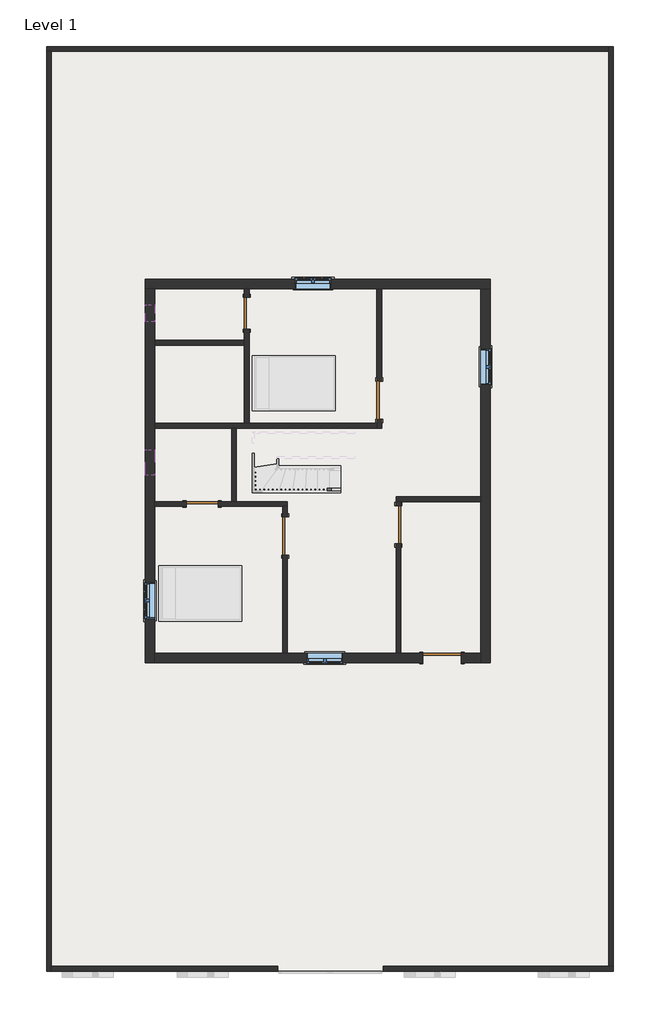
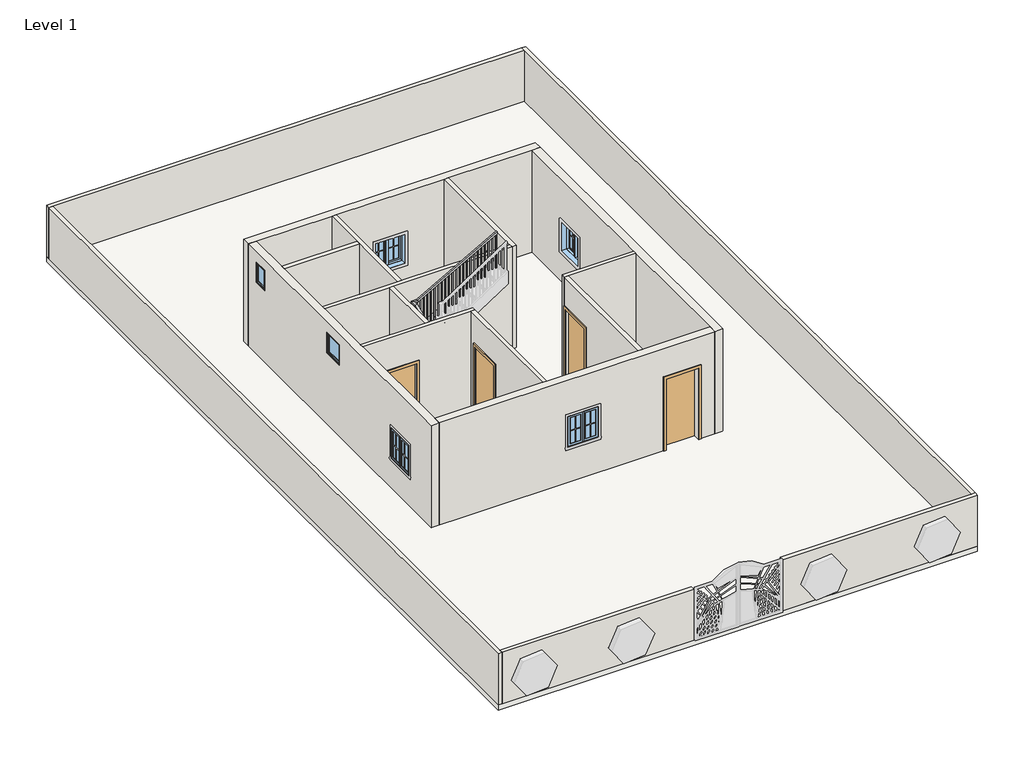
# One storey, part 1 of 2: 18 walls, 6 doors, 6 windows, 1 railing, 1 slab.
"""IFC4 building model written with IfcOpenShell, lengths in millimetres."""

from ifc_helpers import new_model, si_unit, frame, origin, origin_with_axes, place, context, project, spatial, polyline, outline, extrude, faceted_brep, transform, mapped, element, save
from components import door_d8f5dbb5, door_f2b275c1, door_305aa2a5, door_e5f9f3c4, door_0ca8825f, window_aa618e30, window_80340324, window_339605e1

model = new_model("IFC4")

# Units and contexts
model_context = context("Model", 3, world=origin())
ifc_project = project(units=[si_unit("LENGTHUNIT", "METRE", prefix="MILLI")], contexts=[model_context])

# Site, building, storey
site = spatial("IfcSite", under=ifc_project)
building = spatial("IfcBuilding", under=site)
storey = spatial("IfcBuildingStorey", under=building, Name="Level 1", Elevation=0.0)

# Doors
placement = place(None, origin())
door_shape = door_d8f5dbb5(model_context)
element("IfcDoor", 1, ObjectType="Single-Flush : 30\" x 80\"", at=placement, inside=storey, context=model_context, shape_type="MappedRepresentation", body=[
    mapped(door_shape, transform((-2510.1648498, 3958.5558073, 0.0), x_axis=(0.0, 1.0, 0.0), y_axis=(-1.0, 0.0, 0.0), z_axis=(0.0, 0.0, 1.0))),
])
door_2_shape = door_f2b275c1(model_context)
element("IfcDoor", 2, ObjectType="Single-Flush : 30\" x 80\"", at=placement, inside=storey, context=model_context, shape_type="MappedRepresentation", body=[
    mapped(door_2_shape, transform((-3576.9648498, -592.8066927, 0.0), x_axis=(-1.0, 0.0, 0.0), y_axis=(0.0, -1.0, 0.0), z_axis=(0.0, 0.0, 1.0))),
])
door_3_shape = door_305aa2a5(model_context)
element("IfcDoor", 3, ObjectType="Single-Flush : 36\" x 84\"", at=placement, inside=storey, context=model_context, shape_type="MappedRepresentation", body=[
    mapped(door_3_shape, transform((652.1351502, 1883.6933073, 0.0), x_axis=(0.0, -1.0, 0.0), y_axis=(1.0, 0.0, 0.0), z_axis=(0.0, 0.0, 1.0))),
])
element("IfcDoor", 4, ObjectType="Single-Flush : 36\" x 84\"", at=placement, inside=storey, context=model_context, shape_type="MappedRepresentation", body=[
    mapped(door_3_shape, transform((1109.3351502, -1088.1066927, 0.0), x_axis=(0.0, 1.0, 0.0), y_axis=(-1.0, 0.0, 0.0), z_axis=(0.0, 0.0, 1.0))),
])
door_4_shape = door_e5f9f3c4(model_context)
element("IfcDoor", 5, ObjectType="Single-Flush : 36\" x 84\"", at=placement, inside=storey, context=model_context, shape_type="MappedRepresentation", body=[
    mapped(door_4_shape, transform((-1595.7648498, -1354.8066927, 0.0), x_axis=(0.0, 1.0, 0.0), y_axis=(-1.0, 0.0, 0.0), z_axis=(0.0, 0.0, 1.0))),
])
door_5_shape = door_0ca8825f(model_context)
element("IfcDoor", 6, ObjectType="Single-Flush : 36\" x 84\"", at=placement, inside=storey, context=model_context, shape_type="MappedRepresentation", body=[
    mapped(door_5_shape, transform((2147.5601502, -4269.4566927, 0.0), x_axis=(1.0, 0.0, 0.0), y_axis=(0.0, 1.0, 0.0), z_axis=(0.0, 0.0, 1.0))),
])

# Railing
element("IfcRailing", 7, ObjectType="Handrail - Rectangular", at=placement, inside=storey, context=model_context, shape_type="SolidModel", body=[
    faceted_brep([(-264.8831579, -271.8029286, 1083.7333333), (-264.8831579, -271.8029286, 1026.1518622), (-264.8831579, -221.0029286, 1026.1518622), (-264.8831579, -221.0029286, 1083.7333333), (-2203.3957557, -271.8029286, 2118.266441), (-2216.1029055, -271.8029286, 2067.466441), (-2216.1029055, -221.0029286, 2067.466441), (-2203.3957557, -221.0029286, 2118.266441), (-2328.8610857, -271.8029286, 2118.266441), (-2328.8610857, -271.8029286, 2067.466441), (-2278.0610857, -221.0029286, 2067.466441), (-2278.0610857, -221.0029286, 2118.266441), (-2328.8610857, -117.3180853, 2118.266441), (-2328.8610857, -107.2249429, 2067.466441), (-2278.0610857, -107.2249429, 2067.466441), (-2278.0610857, -117.3180853, 2118.266441), (-2328.8610857, 889.2076495, 2534.6648193), (-2328.8610857, 899.300792, 2483.8648193), (-2278.0610857, 899.300792, 2483.8648193), (-2278.0610857, 889.2076495, 2534.6648193), (-2328.8610857, 1080.0895433, 2534.6648193), (-2328.8610857, 1080.0895433, 2483.8648193), (-2278.0610857, 1029.2895433, 2483.8648193), (-2278.0610857, 1029.2895433, 2534.6648193), (-2181.3423106, 1080.0895433, 2534.6648193), (-2168.0744201, 1080.0895433, 2483.8648193), (-2168.0744201, 1029.2895433, 2483.8648193), (-2181.3423106, 1029.2895433, 2534.6648193), (63.4034409, 1080.0895433, 3793.0666667), (63.4034409, 1029.2895433, 3793.0666667), (63.4034409, 1029.2895433, 3734.8287027), (63.4034409, 1080.0895433, 3734.8287027)], [[[0, 1, 2, 3]], [[1, 0, 4, 5]], [[2, 1, 5, 6]], [[3, 2, 6, 7]], [[0, 3, 7, 4]], [[5, 4, 8, 9]], [[6, 5, 9, 10]], [[7, 6, 10, 11]], [[4, 7, 11, 8]], [[9, 8, 12, 13]], [[10, 9, 13, 14]], [[11, 10, 14, 15]], [[8, 11, 15, 12]], [[13, 12, 16, 17]], [[14, 13, 17, 18]], [[15, 14, 18, 19]], [[12, 15, 19, 16]], [[17, 16, 20, 21]], [[18, 17, 21, 22]], [[19, 18, 22, 23]], [[16, 19, 23, 20]], [[21, 20, 24, 25]], [[22, 21, 25, 26]], [[23, 22, 26, 27]], [[20, 23, 27, 24]], [[28, 29, 30, 31]], [[25, 24, 28, 31]], [[26, 25, 31, 30]], [[27, 26, 30, 29]], [[24, 27, 29, 28]]]),
    extrude(outline(polyline([(3712.6348603, 23.8139143), (2709.3333333, 23.8139143), (2709.3333333, 42.8639143), (3723.3142681, 42.8639143), (3712.6348603, 23.8139143)])), frame((0.0, 1045.1645433, 0.0), z_axis=(0.0, 1.0, 0.0), x_axis=(0.0, 0.0, 1.0)), (0.0, 0.0, 1.0), 19.05),
    extrude(outline(polyline([(3655.678019, -77.7860857), (2709.3333333, -77.7860857), (2709.3333333, -58.7360857), (3666.3574267, -58.7360857), (3655.678019, -77.7860857)])), frame((0.0, 1045.1645433, 0.0), z_axis=(0.0, 1.0, 0.0), x_axis=(0.0, 0.0, 1.0)), (0.0, 0.0, 1.0), 19.05),
    extrude(outline(polyline([(3598.7211776, -179.3860857), (2709.3333333, -179.3860857), (2709.3333333, -160.3360857), (3609.4005853, -160.3360857), (3598.7211776, -179.3860857)])), frame((0.0, 1045.1645433, 0.0), z_axis=(0.0, 1.0, 0.0), x_axis=(0.0, 0.0, 1.0)), (0.0, 0.0, 1.0), 19.05),
    extrude(outline(polyline([(3541.7643362, -280.9860857), (2540.0, -280.9860857), (2540.0, -261.9360857), (3552.443744, -261.9360857), (3541.7643362, -280.9860857)])), frame((0.0, 1045.1645433, 0.0), z_axis=(0.0, 1.0, 0.0), x_axis=(0.0, 0.0, 1.0)), (0.0, 0.0, 1.0), 19.05),
    extrude(outline(polyline([(3484.8074948, -382.5860857), (2540.0, -382.5860857), (2540.0, -363.5360857), (3495.4869026, -363.5360857), (3484.8074948, -382.5860857)])), frame((0.0, 1045.1645433, 0.0), z_axis=(0.0, 1.0, 0.0), x_axis=(0.0, 0.0, 1.0)), (0.0, 0.0, 1.0), 19.05),
    extrude(outline(polyline([(3427.8506535, -484.1860857), (2540.0, -484.1860857), (2540.0, -465.1360857), (3438.5300612, -465.1360857), (3427.8506535, -484.1860857)])), frame((0.0, 1045.1645433, 0.0), z_axis=(0.0, 1.0, 0.0), x_axis=(0.0, 0.0, 1.0)), (0.0, 0.0, 1.0), 19.05),
    extrude(outline(polyline([(3370.8938121, -585.7860857), (2370.6666667, -585.7860857), (2370.6666667, -566.7360857), (3381.5732198, -566.7360857), (3370.8938121, -585.7860857)])), frame((0.0, 1045.1645433, 0.0), z_axis=(0.0, 1.0, 0.0), x_axis=(0.0, 0.0, 1.0)), (0.0, 0.0, 1.0), 19.05),
    extrude(outline(polyline([(3313.9369707, -687.3860857), (2370.6666667, -687.3860857), (2370.6666667, -668.3360857), (3324.6163785, -668.3360857), (3313.9369707, -687.3860857)])), frame((0.0, 1045.1645433, 0.0), z_axis=(0.0, 1.0, 0.0), x_axis=(0.0, 0.0, 1.0)), (0.0, 0.0, 1.0), 19.05),
    extrude(outline(polyline([(3256.9801293, -788.9860857), (2370.6666667, -788.9860857), (2370.6666667, -769.9360857), (3267.6595371, -769.9360857), (3256.9801293, -788.9860857)])), frame((0.0, 1045.1645433, 0.0), z_axis=(0.0, 1.0, 0.0), x_axis=(0.0, 0.0, 1.0)), (0.0, 0.0, 1.0), 19.05),
    extrude(outline(polyline([(3200.023288, -890.5860857), (2201.3333333, -890.5860857), (2201.3333333, -871.5360857), (3210.7026957, -871.5360857), (3200.023288, -890.5860857)])), frame((0.0, 1045.1645433, 0.0), z_axis=(0.0, 1.0, 0.0), x_axis=(0.0, 0.0, 1.0)), (0.0, 0.0, 1.0), 19.05),
    extrude(outline(polyline([(3143.0664466, -992.1860857), (2201.3333333, -992.1860857), (2201.3333333, -973.1360857), (3153.7458543, -973.1360857), (3143.0664466, -992.1860857)])), frame((0.0, 1045.1645433, 0.0), z_axis=(0.0, 1.0, 0.0), x_axis=(0.0, 0.0, 1.0)), (0.0, 0.0, 1.0), 19.05),
    extrude(outline(polyline([(3086.1096052, -1093.7860857), (2032.0, -1093.7860857), (2032.0, -1074.7360857), (3096.789013, -1074.7360857), (3086.1096052, -1093.7860857)])), frame((0.0, 1045.1645433, 0.0), z_axis=(0.0, 1.0, 0.0), x_axis=(0.0, 0.0, 1.0)), (0.0, 0.0, 1.0), 19.05),
    extrude(outline(polyline([(3029.1527638, -1195.3860857), (2032.0, -1195.3860857), (2032.0, -1176.3360857), (3039.8321716, -1176.3360857), (3029.1527638, -1195.3860857)])), frame((0.0, 1045.1645433, 0.0), z_axis=(0.0, 1.0, 0.0), x_axis=(0.0, 0.0, 1.0)), (0.0, 0.0, 1.0), 19.05),
    extrude(outline(polyline([(2972.1959225, -1296.9860857), (2032.0, -1296.9860857), (2032.0, -1277.9360857), (2982.8753302, -1277.9360857), (2972.1959225, -1296.9860857)])), frame((0.0, 1045.1645433, 0.0), z_axis=(0.0, 1.0, 0.0), x_axis=(0.0, 0.0, 1.0)), (0.0, 0.0, 1.0), 19.05),
    extrude(outline(polyline([(2915.2390811, -1398.5860857), (1862.6666667, -1398.5860857), (1862.6666667, -1379.5360857), (2925.9184889, -1379.5360857), (2915.2390811, -1398.5860857)])), frame((0.0, 1045.1645433, 0.0), z_axis=(0.0, 1.0, 0.0), x_axis=(0.0, 0.0, 1.0)), (0.0, 0.0, 1.0), 19.05),
    extrude(outline(polyline([(2858.2822397, -1500.1860857), (1862.6666667, -1500.1860857), (1862.6666667, -1481.1360857), (2868.9616475, -1481.1360857), (2858.2822397, -1500.1860857)])), frame((0.0, 1045.1645433, 0.0), z_axis=(0.0, 1.0, 0.0), x_axis=(0.0, 0.0, 1.0)), (0.0, 0.0, 1.0), 19.05),
    extrude(outline(polyline([(2801.3253983, -1601.7860857), (1862.6666667, -1601.7860857), (1862.6666667, -1582.7360857), (2812.0048061, -1582.7360857), (2801.3253983, -1601.7860857)])), frame((0.0, 1045.1645433, 0.0), z_axis=(0.0, 1.0, 0.0), x_axis=(0.0, 0.0, 1.0)), (0.0, 0.0, 1.0), 19.05),
    extrude(outline(polyline([(2744.368557, -1703.3860857), (1693.3333333, -1703.3860857), (1693.3333333, -1684.3360857), (2755.0479647, -1684.3360857), (2744.368557, -1703.3860857)])), frame((0.0, 1045.1645433, 0.0), z_axis=(0.0, 1.0, 0.0), x_axis=(0.0, 0.0, 1.0)), (0.0, 0.0, 1.0), 19.05),
    extrude(outline(polyline([(2687.4117156, -1804.9860857), (1693.3333333, -1804.9860857), (1693.3333333, -1785.9360857), (2698.0911234, -1785.9360857), (2687.4117156, -1804.9860857)])), frame((0.0, 1045.1645433, 0.0), z_axis=(0.0, 1.0, 0.0), x_axis=(0.0, 0.0, 1.0)), (0.0, 0.0, 1.0), 19.05),
    extrude(outline(polyline([(2630.4548742, -1906.5860857), (1693.3333333, -1906.5860857), (1693.3333333, -1887.5360857), (2641.134282, -1887.5360857), (2630.4548742, -1906.5860857)])), frame((0.0, 1045.1645433, 0.0), z_axis=(0.0, 1.0, 0.0), x_axis=(0.0, 0.0, 1.0)), (0.0, 0.0, 1.0), 19.05),
    extrude(outline(polyline([(2573.4980329, -2008.1860857), (1693.3333333, -2008.1860857), (1693.3333333, -1989.1360857), (2584.1774406, -1989.1360857), (2573.4980329, -2008.1860857)])), frame((0.0, 1045.1645433, 0.0), z_axis=(0.0, 1.0, 0.0), x_axis=(0.0, 0.0, 1.0)), (0.0, 0.0, 1.0), 19.05),
    extrude(outline(polyline([(2516.5411915, -2109.7860857), (1524.0, -2109.7860857), (1524.0, -2090.7360857), (2527.2205992, -2090.7360857), (2516.5411915, -2109.7860857)])), frame((0.0, 1045.1645433, 0.0), z_axis=(0.0, 1.0, 0.0), x_axis=(0.0, 0.0, 1.0)), (0.0, 0.0, 1.0), 19.05),
    extrude(outline(polyline([(-2211.3860857, 1064.2145433), (-2192.3360857, 1064.2145433), (-2192.3360857, 1045.1645433), (-2211.3860857, 1045.1645433), (-2211.3860857, 1064.2145433)])), frame((0.0, 0.0, 1524.0), z_axis=(0.0, 0.0, 1.0), x_axis=(1.0, 0.0, 0.0)), (0.0, 0.0, 1.0), 959.8648193),
    extrude(outline(polyline([(-2312.9860857, 963.2720714), (-2312.9860857, 982.3220714), (-2293.9360857, 982.3220714), (-2293.9360857, 963.2720714), (-2312.9860857, 963.2720714)])), frame((0.0, 0.0, 1524.0), z_axis=(0.0, 0.0, 1.0), x_axis=(1.0, 0.0, 0.0)), (0.0, 0.0, 1.0), 959.8648193),
    extrude(outline(polyline([(880.7220714, 2476.1788269), (880.7220714, 1524.0), (861.6720714, 1524.0), (861.6720714, 2468.2978669), (880.7220714, 2476.1788269)])), frame((-2312.9860857, 0.0, 0.0), z_axis=(1.0, 0.0, 0.0), x_axis=(0.0, 1.0, 0.0)), (0.0, 0.0, 1.0), 19.05),
    extrude(outline(polyline([(779.1220714, 2434.14704), (779.1220714, 1524.0), (760.0720714, 1524.0), (760.0720714, 2426.2660799), (779.1220714, 2434.14704)])), frame((-2312.9860857, 0.0, 0.0), z_axis=(1.0, 0.0, 0.0), x_axis=(0.0, 1.0, 0.0)), (0.0, 0.0, 1.0), 19.05),
    extrude(outline(polyline([(677.5220714, 2392.115253), (677.5220714, 1524.0), (658.4720714, 1524.0), (658.4720714, 2384.234293), (677.5220714, 2392.115253)])), frame((-2312.9860857, 0.0, 0.0), z_axis=(1.0, 0.0, 0.0), x_axis=(0.0, 1.0, 0.0)), (0.0, 0.0, 1.0), 19.05),
    extrude(outline(polyline([(575.9220714, 2350.0834661), (575.9220714, 1354.6666667), (556.8720714, 1354.6666667), (556.8720714, 2342.202506), (575.9220714, 2350.0834661)])), frame((-2312.9860857, 0.0, 0.0), z_axis=(1.0, 0.0, 0.0), x_axis=(0.0, 1.0, 0.0)), (0.0, 0.0, 1.0), 19.05),
    extrude(outline(polyline([(474.3220714, 2308.0516792), (474.3220714, 1354.6666667), (455.2720714, 1354.6666667), (455.2720714, 2300.1707191), (474.3220714, 2308.0516792)])), frame((-2312.9860857, 0.0, 0.0), z_axis=(1.0, 0.0, 0.0), x_axis=(0.0, 1.0, 0.0)), (0.0, 0.0, 1.0), 19.05),
    extrude(outline(polyline([(372.7220714, 2266.0198922), (372.7220714, 1354.6666667), (353.6720714, 1354.6666667), (353.6720714, 2258.1389322), (372.7220714, 2266.0198922)])), frame((-2312.9860857, 0.0, 0.0), z_axis=(1.0, 0.0, 0.0), x_axis=(0.0, 1.0, 0.0)), (0.0, 0.0, 1.0), 19.05),
    extrude(outline(polyline([(271.1220714, 2223.9881053), (271.1220714, 1354.6666667), (252.0720714, 1354.6666667), (252.0720714, 2216.1071452), (271.1220714, 2223.9881053)])), frame((-2312.9860857, 0.0, 0.0), z_axis=(1.0, 0.0, 0.0), x_axis=(0.0, 1.0, 0.0)), (0.0, 0.0, 1.0), 19.05),
    extrude(outline(polyline([(169.5220714, 2181.9563183), (169.5220714, 1185.3333333), (150.4720714, 1185.3333333), (150.4720714, 2174.0753583), (169.5220714, 2181.9563183)])), frame((-2312.9860857, 0.0, 0.0), z_axis=(1.0, 0.0, 0.0), x_axis=(0.0, 1.0, 0.0)), (0.0, 0.0, 1.0), 19.05),
    extrude(outline(polyline([(67.9220714, 2139.9245314), (67.9220714, 1185.3333333), (48.8720714, 1185.3333333), (48.8720714, 2132.0435714), (67.9220714, 2139.9245314)])), frame((-2312.9860857, 0.0, 0.0), z_axis=(1.0, 0.0, 0.0), x_axis=(0.0, 1.0, 0.0)), (0.0, 0.0, 1.0), 19.05),
    extrude(outline(polyline([(-33.6779286, 2097.8927445), (-33.6779286, 1185.3333333), (-52.7279286, 1185.3333333), (-52.7279286, 2090.0117844), (-33.6779286, 2097.8927445)])), frame((-2312.9860857, 0.0, 0.0), z_axis=(1.0, 0.0, 0.0), x_axis=(0.0, 1.0, 0.0)), (0.0, 0.0, 1.0), 19.05),
    extrude(outline(polyline([(-2312.9860857, -154.3279286), (-2312.9860857, -135.2779286), (-2293.9360857, -135.2779286), (-2293.9360857, -154.3279286), (-2312.9860857, -154.3279286)])), frame((0.0, 0.0, 1185.3333333), z_axis=(0.0, 0.0, 1.0), x_axis=(1.0, 0.0, 0.0)), (0.0, 0.0, 1.0), 882.1331077),
    extrude(outline(polyline([(-2287.3581579, -255.9279286), (-2306.4081579, -255.9279286), (-2306.4081579, -236.8779286), (-2287.3581579, -236.8779286), (-2287.3581579, -255.9279286)])), frame((0.0, 0.0, 1185.3333333), z_axis=(0.0, 0.0, 1.0), x_axis=(1.0, 0.0, 0.0)), (0.0, 0.0, 1.0), 882.1331077),
    extrude(outline(polyline([(2061.4387317, -2204.8081579), (1185.3333333, -2204.8081579), (1185.3333333, -2185.7581579), (2051.2722486, -2185.7581579), (2061.4387317, -2204.8081579)])), frame((0.0, -255.9279286, 0.0), z_axis=(0.0, 1.0, 0.0), x_axis=(0.0, 0.0, 1.0)), (0.0, 0.0, 1.0), 19.05),
    extrude(outline(polyline([(2007.2174882, -2103.2081579), (1016.0, -2103.2081579), (1016.0, -2084.1581579), (1997.051005, -2084.1581579), (2007.2174882, -2103.2081579)])), frame((0.0, -255.9279286, 0.0), z_axis=(0.0, 1.0, 0.0), x_axis=(0.0, 0.0, 1.0)), (0.0, 0.0, 1.0), 19.05),
    extrude(outline(polyline([(1952.9962446, -2001.6081579), (1016.0, -2001.6081579), (1016.0, -1982.5581579), (1942.8297614, -1982.5581579), (1952.9962446, -2001.6081579)])), frame((0.0, -255.9279286, 0.0), z_axis=(0.0, 1.0, 0.0), x_axis=(0.0, 0.0, 1.0)), (0.0, 0.0, 1.0), 19.05),
    extrude(outline(polyline([(1898.7332033, -1900.0081579), (1016.0, -1900.0081579), (1016.0, -1880.9581579), (1888.6645789, -1880.9581579), (1898.7332033, -1900.0081579)])), frame((0.0, -255.9279286, 0.0), z_axis=(0.0, 1.0, 0.0), x_axis=(0.0, 0.0, 1.0)), (0.0, 0.0, 1.0), 19.05),
    extrude(outline(polyline([(1844.5537574, -1798.4081579), (1016.0, -1798.4081579), (1016.0, -1779.3581579), (1834.3872743, -1779.3581579), (1844.5537574, -1798.4081579)])), frame((0.0, -255.9279286, 0.0), z_axis=(0.0, 1.0, 0.0), x_axis=(0.0, 0.0, 1.0)), (0.0, 0.0, 1.0), 19.05),
    extrude(outline(polyline([(1790.2644227, -1696.8081579), (846.6666667, -1696.8081579), (846.6666667, -1677.7581579), (1780.1957983, -1677.7581579), (1790.2644227, -1696.8081579)])), frame((0.0, -255.9279286, 0.0), z_axis=(0.0, 1.0, 0.0), x_axis=(0.0, 0.0, 1.0)), (0.0, 0.0, 1.0), 19.05),
    extrude(outline(polyline([(1736.1112703, -1595.2081579), (846.6666667, -1595.2081579), (846.6666667, -1576.1581579), (1725.9447871, -1576.1581579), (1736.1112703, -1595.2081579)])), frame((0.0, -255.9279286, 0.0), z_axis=(0.0, 1.0, 0.0), x_axis=(0.0, 0.0, 1.0)), (0.0, 0.0, 1.0), 19.05),
    extrude(outline(polyline([(1681.8900267, -1493.6081579), (846.6666667, -1493.6081579), (846.6666667, -1474.5581579), (1671.7235435, -1474.5581579), (1681.8900267, -1493.6081579)])), frame((0.0, -255.9279286, 0.0), z_axis=(0.0, 1.0, 0.0), x_axis=(0.0, 0.0, 1.0)), (0.0, 0.0, 1.0), 19.05),
    extrude(outline(polyline([(1627.6687831, -1392.0081579), (677.3333333, -1392.0081579), (677.3333333, -1372.9581579), (1617.5023, -1372.9581579), (1627.6687831, -1392.0081579)])), frame((0.0, -255.9279286, 0.0), z_axis=(0.0, 1.0, 0.0), x_axis=(0.0, 0.0, 1.0)), (0.0, 0.0, 1.0), 19.05),
    extrude(outline(polyline([(1573.4475396, -1290.4081579), (677.3333333, -1290.4081579), (677.3333333, -1271.3581579), (1563.2810564, -1271.3581579), (1573.4475396, -1290.4081579)])), frame((0.0, -255.9279286, 0.0), z_axis=(0.0, 1.0, 0.0), x_axis=(0.0, 0.0, 1.0)), (0.0, 0.0, 1.0), 19.05),
    extrude(outline(polyline([(1519.226296, -1188.8081579), (677.3333333, -1188.8081579), (677.3333333, -1169.7581579), (1509.0598128, -1169.7581579), (1519.226296, -1188.8081579)])), frame((0.0, -255.9279286, 0.0), z_axis=(0.0, 1.0, 0.0), x_axis=(0.0, 0.0, 1.0)), (0.0, 0.0, 1.0), 19.05),
    extrude(outline(polyline([(1465.0050524, -1087.2081579), (508.0, -1087.2081579), (508.0, -1068.1581579), (1454.8385692, -1068.1581579), (1465.0050524, -1087.2081579)])), frame((0.0, -255.9279286, 0.0), z_axis=(0.0, 1.0, 0.0), x_axis=(0.0, 0.0, 1.0)), (0.0, 0.0, 1.0), 19.05),
    extrude(outline(polyline([(1410.7838088, -985.6081579), (508.0, -985.6081579), (508.0, -966.5581579), (1400.6173257, -966.5581579), (1410.7838088, -985.6081579)])), frame((0.0, -255.9279286, 0.0), z_axis=(0.0, 1.0, 0.0), x_axis=(0.0, 0.0, 1.0)), (0.0, 0.0, 1.0), 19.05),
    extrude(outline(polyline([(1356.5625653, -884.0081579), (508.0, -884.0081579), (508.0, -864.9581579), (1346.3960821, -864.9581579), (1356.5625653, -884.0081579)])), frame((0.0, -255.9279286, 0.0), z_axis=(0.0, 1.0, 0.0), x_axis=(0.0, 0.0, 1.0)), (0.0, 0.0, 1.0), 19.05),
    extrude(outline(polyline([(1302.3413217, -782.4081579), (338.6666667, -782.4081579), (338.6666667, -763.3581579), (1292.1748385, -763.3581579), (1302.3413217, -782.4081579)])), frame((0.0, -255.9279286, 0.0), z_axis=(0.0, 1.0, 0.0), x_axis=(0.0, 0.0, 1.0)), (0.0, 0.0, 1.0), 19.05),
    extrude(outline(polyline([(1248.1200781, -680.8081579), (338.6666667, -680.8081579), (338.6666667, -661.7581579), (1237.9535949, -661.7581579), (1248.1200781, -680.8081579)])), frame((0.0, -255.9279286, 0.0), z_axis=(0.0, 1.0, 0.0), x_axis=(0.0, 0.0, 1.0)), (0.0, 0.0, 1.0), 19.05),
    extrude(outline(polyline([(1193.8988345, -579.2081579), (338.6666667, -579.2081579), (338.6666667, -560.1581579), (1183.7323514, -560.1581579), (1193.8988345, -579.2081579)])), frame((0.0, -255.9279286, 0.0), z_axis=(0.0, 1.0, 0.0), x_axis=(0.0, 0.0, 1.0)), (0.0, 0.0, 1.0), 19.05),
    extrude(outline(polyline([(1139.677591, -477.6081579), (169.3333333, -477.6081579), (169.3333333, -458.5581579), (1129.5111078, -458.5581579), (1139.677591, -477.6081579)])), frame((0.0, -255.9279286, 0.0), z_axis=(0.0, 1.0, 0.0), x_axis=(0.0, 0.0, 1.0)), (0.0, 0.0, 1.0), 19.05),
    extrude(outline(polyline([(1085.4563474, -376.0081579), (169.3333333, -376.0081579), (169.3333333, -356.9581579), (1075.2898642, -356.9581579), (1085.4563474, -376.0081579)])), frame((0.0, -255.9279286, 0.0), z_axis=(0.0, 1.0, 0.0), x_axis=(0.0, 0.0, 1.0)), (0.0, 0.0, 1.0), 19.05),
    extrude(outline(polyline([(-2312.9860857, 1045.1645433), (-2312.9860857, 1064.2145433), (-2293.9360857, 1064.2145433), (-2293.9360857, 1045.1645433), (-2312.9860857, 1045.1645433)])), frame((0.0, 0.0, 1524.0), z_axis=(0.0, 0.0, 1.0), x_axis=(1.0, 0.0, 0.0)), (0.0, 0.0, 1.0), 959.8648193),
    extrude(outline(polyline([(-2293.9360857, -255.9279286), (-2312.9860857, -255.9279286), (-2312.9860857, -236.8779286), (-2293.9360857, -236.8779286), (-2293.9360857, -255.9279286)])), frame((0.0, 0.0, 1185.3333333), z_axis=(0.0, 0.0, 1.0), x_axis=(1.0, 0.0, 0.0)), (0.0, 0.0, 1.0), 882.1331077),
    extrude(outline(polyline([(3724.149295, 44.3534409), (2709.3333333, 44.3534409), (2709.3333333, 63.4034409), (3734.8287027, 63.4034409), (3724.149295, 44.3534409)])), frame((0.0, 1045.1645433, 0.0), z_axis=(0.0, 1.0, 0.0), x_axis=(0.0, 0.0, 1.0)), (0.0, 0.0, 1.0), 19.05),
    extrude(outline(polyline([(1036.3428896, -283.9331579), (169.3333333, -283.9331579), (169.3333333, -264.8831579), (1026.2742652, -264.8831579), (1036.3428896, -283.9331579)])), frame((0.0, -255.9279286, 0.0), z_axis=(0.0, 1.0, 0.0), x_axis=(0.0, 0.0, 1.0)), (0.0, 0.0, 1.0), 19.05),
])

# Slab
element("IfcSlab", 8, ObjectType="Generic - 12\"", at=placement, inside=storey, context=model_context, shape_type="SweptSolid", body=[
    extrude(outline(polyline([(6238.3832079, 10322.884496), (6238.3832079, -11737.015504), (-7287.1167921, -11737.015504), (-7287.1167921, 10322.884496), (6238.3832079, 10322.884496)])), frame((0.0, 0.0, -152.4), z_axis=(0.0, 0.0, 1.0), x_axis=(1.0, 0.0, 0.0)), (0.0, 0.0, 1.0), 152.4),
])

# Walls
element("IfcWall", 9, ObjectType="WALL4.5\"", at=placement, inside=storey, context=model_context, shape_type="SweptSolid", body=[
    extrude(outline(polyline([(-2567.3148498, 3198.1433073), (-4700.9148498, 3198.1433073), (-4700.9148498, 3312.4433073), (-2567.3148498, 3312.4433073), (-2567.3148498, 3198.1433073)])), origin_with_axes(), (0.0, 0.0, 1.0), 3048.0),
])
element("IfcWall", 10, ObjectType="WALL4.5\"", at=placement, inside=storey, context=model_context, shape_type="Brep", body=[
    faceted_brep([(-2567.3148498, 4547.5183073, 0.0), (-2567.3148498, 4339.5558073, 0.0), (-2567.3148498, 4339.5558073, 2032.0), (-2567.3148498, 3577.5558073, 2032.0), (-2567.3148498, 3577.5558073, 0.0), (-2567.3148498, 3312.4433073, 0.0), (-2567.3148498, 3198.1433073, 0.0), (-2567.3148498, 1331.2433073, 0.0), (-2567.3148498, 1331.2433073, 3048.0), (-2567.3148498, 3198.1433073, 3048.0), (-2567.3148498, 3312.4433073, 3048.0), (-2567.3148498, 4547.5183073, 3048.0), (-2453.0148498, 4339.5558073, 2032.0), (-2453.0148498, 4339.5558073, 0.0), (-2453.0148498, 4547.5183073, 0.0), (-2453.0148498, 4547.5183073, 3048.0), (-2453.0148498, 1331.2433073, 3048.0), (-2453.0148498, 1331.2433073, 0.0), (-2453.0148498, 3577.5558073, 0.0), (-2453.0148498, 3577.5558073, 2032.0)], [[[0, 1, 2, 3, 4, 5, 6, 7, 8, 9, 10, 11]], [[12, 13, 14, 15, 16, 17, 18, 19]], [[18, 17, 7, 6, 5, 4]], [[14, 13, 1, 0]], [[0, 11, 15, 14]], [[8, 7, 17, 16]], [[2, 1, 13, 12]], [[3, 2, 12, 19]], [[4, 3, 19, 18]], [[11, 10, 9, 8, 16, 15]]]),
])
element("IfcWall", 11, ObjectType="WALL4.5\"", at=placement, inside=storey, context=model_context, shape_type="Brep", body=[
    faceted_brep([(594.9851502, 1426.4933073, 2133.6), (594.9851502, 1426.4933073, 0.0), (594.9851502, 1331.2433073, 0.0), (594.9851502, 1216.9433073, 0.0), (594.9851502, 1216.9433073, 3048.0), (594.9851502, 1331.2433073, 3048.0), (594.9851502, 4547.5183073, 3048.0), (594.9851502, 4547.5183073, 0.0), (594.9851502, 2340.8933073, 0.0), (594.9851502, 2340.8933073, 2133.6), (709.2851502, 1216.9433073, 0.0), (709.2851502, 1426.4933073, 0.0), (709.2851502, 1426.4933073, 2133.6), (709.2851502, 2340.8933073, 2133.6), (709.2851502, 2340.8933073, 0.0), (709.2851502, 4547.5183073, 0.0), (709.2851502, 4547.5183073, 3048.0), (709.2851502, 1216.9433073, 3048.0)], [[[0, 1, 2, 3, 4, 5, 6, 7, 8, 9]], [[10, 11, 12, 13, 14, 15, 16, 17]], [[8, 7, 15, 14]], [[3, 2, 1, 11, 10]], [[7, 6, 16, 15]], [[4, 3, 10, 17]], [[12, 11, 1, 0]], [[13, 12, 0, 9]], [[14, 13, 9, 8]], [[6, 5, 4, 17, 16]]]),
])
element("IfcWall", 12, ObjectType="WALL4.5\"", at=placement, inside=storey, context=model_context, shape_type="Brep", body=[
    faceted_brep([(-4700.9148498, 1216.9433073, 0.0), (-2872.1148498, 1216.9433073, 0.0), (-2757.8148498, 1216.9433073, 0.0), (594.9851502, 1216.9433073, 0.0), (594.9851502, 1216.9433073, 3048.0), (-2757.8148498, 1216.9433073, 3048.0), (-2872.1148498, 1216.9433073, 3048.0), (-4700.9148498, 1216.9433073, 3048.0), (-4700.9148498, 1331.2433073, 0.0), (-4700.9148498, 1331.2433073, 3048.0), (-2567.3148498, 1331.2433073, 3048.0), (-2453.0148498, 1331.2433073, 3048.0), (594.9851502, 1331.2433073, 3048.0), (594.9851502, 1331.2433073, 0.0), (-2453.0148498, 1331.2433073, 0.0), (-2567.3148498, 1331.2433073, 0.0)], [[[0, 1, 2, 3, 4, 5, 6, 7]], [[8, 9, 10, 11, 12, 13, 14, 15]], [[3, 2, 1, 0, 8, 15, 14, 13]], [[4, 3, 13, 12]], [[0, 7, 9, 8]], [[7, 6, 5, 4, 12, 11, 10, 9]]]),
])
element("IfcWall", 13, ObjectType="WALL4.5\"", at=placement, inside=storey, context=model_context, shape_type="SweptSolid", body=[
    extrude(outline(polyline([(-2872.1148498, -535.6566927), (-2872.1148498, 1216.9433073), (-2757.8148498, 1216.9433073), (-2757.8148498, -535.6566927), (-2872.1148498, -535.6566927)])), origin_with_axes(), (0.0, 0.0, 1.0), 3048.0),
])
element("IfcWall", 14, ObjectType="WALL4.5\"", at=placement, inside=storey, context=model_context, shape_type="Brep", body=[
    faceted_brep([(-4700.9148498, -649.9566927, 0.0), (-3957.9648498, -649.9566927, 0.0), (-3957.9648498, -649.9566927, 2032.0), (-3195.9648498, -649.9566927, 2032.0), (-3195.9648498, -649.9566927, 0.0), (-1652.9148498, -649.9566927, 0.0), (-1538.6148498, -649.9566927, 0.0), (-1538.6148498, -649.9566927, 3048.0), (-1652.9148498, -649.9566927, 3048.0), (-4700.9148498, -649.9566927, 3048.0), (-3957.9648498, -535.6566927, 2032.0), (-3957.9648498, -535.6566927, 0.0), (-4700.9148498, -535.6566927, 0.0), (-4700.9148498, -535.6566927, 3048.0), (-2872.1148498, -535.6566927, 3048.0), (-2757.8148498, -535.6566927, 3048.0), (-1538.6148498, -535.6566927, 3048.0), (-1538.6148498, -535.6566927, 0.0), (-2757.8148498, -535.6566927, 0.0), (-2872.1148498, -535.6566927, 0.0), (-3195.9648498, -535.6566927, 0.0), (-3195.9648498, -535.6566927, 2032.0)], [[[0, 1, 2, 3, 4, 5, 6, 7, 8, 9]], [[10, 11, 12, 13, 14, 15, 16, 17, 18, 19, 20, 21]], [[12, 11, 1, 0]], [[20, 19, 18, 17, 6, 5, 4]], [[7, 6, 17, 16]], [[0, 9, 13, 12]], [[2, 1, 11, 10]], [[3, 2, 10, 21]], [[4, 3, 21, 20]], [[9, 8, 7, 16, 15, 14, 13]]]),
])
element("IfcWall", 15, ObjectType="WALL4.5\"", at=placement, inside=storey, context=model_context, shape_type="Brep", body=[
    faceted_brep([(3071.4851502, -421.3566927, 0.0), (1052.1851502, -421.3566927, 0.0), (1052.1851502, -421.3566927, 3048.0), (3071.4851502, -421.3566927, 3048.0), (3071.4851502, -535.6566927, 0.0), (3071.4851502, -535.6566927, 3048.0), (1166.4851502, -535.6566927, 3048.0), (1052.1851502, -535.6566927, 3048.0), (1052.1851502, -535.6566927, 0.0), (1166.4851502, -535.6566927, 0.0)], [[[0, 1, 2, 3]], [[4, 5, 6, 7, 8, 9]], [[1, 0, 4, 9, 8]], [[0, 3, 5, 4]], [[2, 1, 8, 7]], [[3, 2, 7, 6, 5]]]),
])
element("IfcWall", 16, ObjectType="WALL4.5\"", at=placement, inside=storey, context=model_context, shape_type="SweptSolid", body=[
    extrude(outline(polyline([(-535.6566927, 0.0), (-630.9066927, 0.0), (-630.9066927, 2133.6), (-1545.3066927, 2133.6), (-1545.3066927, 0.0), (-4155.1566927, 0.0), (-4155.1566927, 3048.0), (-535.6566927, 3048.0), (-535.6566927, 0.0)])), frame((1052.1851502, 0.0, 0.0), z_axis=(1.0, 0.0, 0.0), x_axis=(0.0, 1.0, 0.0)), (0.0, 0.0, 1.0), 114.3),
])
element("IfcWall", 17, ObjectType="WALL4.5\"", at=placement, inside=storey, context=model_context, shape_type="SweptSolid", body=[
    extrude(outline(polyline([(-649.9566927, 0.0), (-897.6066927, 0.0), (-897.6066927, 2133.6), (-1812.0066927, 2133.6), (-1812.0066927, 0.0), (-4155.1566927, 0.0), (-4155.1566927, 3048.0), (-649.9566927, 3048.0), (-649.9566927, 0.0)])), frame((-1652.9148498, 0.0, 0.0), z_axis=(1.0, 0.0, 0.0), x_axis=(0.0, 1.0, 0.0)), (0.0, 0.0, 1.0), 114.3),
])
element("IfcWall", 18, ObjectType="WALL4.5\"", at=placement, inside=storey, context=model_context, shape_type="Brep", body=[
    faceted_brep([(-7287.1167921, 10208.584496, 0.0), (-7172.8167921, 10208.584496, 0.0), (6124.0832079, 10208.584496, 0.0), (6124.0832079, 10208.584496, 1524.0), (-7172.8167921, 10208.584496, 1524.0), (-7287.1167921, 10208.584496, 1524.0), (-7287.1167921, 10322.884496, 0.0), (-7287.1167921, 10322.884496, 1524.0), (6124.0832079, 10322.884496, 1524.0), (6124.0832079, 10322.884496, 0.0)], [[[0, 1, 2, 3, 4, 5]], [[6, 7, 8, 9]], [[2, 1, 0, 6, 9]], [[5, 4, 3, 8, 7]], [[0, 5, 7, 6]], [[3, 2, 9, 8]]]),
])
element("IfcWall", 19, ObjectType="WALL4.5\"", at=placement, inside=storey, context=model_context, shape_type="Brep", body=[
    faceted_brep([(-7172.8167921, -11737.015504, 0.0), (-7172.8167921, -11622.715504, 0.0), (-7172.8167921, 10208.584496, 0.0), (-7172.8167921, 10208.584496, 1524.0), (-7172.8167921, -11622.715504, 1524.0), (-7172.8167921, -11737.015504, 1524.0), (-7287.1167921, -11737.015504, 0.0), (-7287.1167921, -11737.015504, 1524.0), (-7287.1167921, 10208.584496, 1524.0), (-7287.1167921, 10208.584496, 0.0)], [[[0, 1, 2, 3, 4, 5]], [[6, 7, 8, 9]], [[2, 1, 0, 6, 9]], [[5, 4, 3, 8, 7]], [[0, 5, 7, 6]], [[3, 2, 9, 8]]]),
])
element("IfcWall", 20, ObjectType="WALL4.5\"", at=placement, inside=storey, context=model_context, shape_type="Brep", body=[
    faceted_brep([(6238.3832079, -11622.715504, 0.0), (6124.0832079, -11622.715504, 0.0), (745.6332079, -11622.715504, 0.0), (745.6332079, -11622.715504, 1524.0), (6124.0832079, -11622.715504, 1524.0), (6238.3832079, -11622.715504, 1524.0), (6238.3832079, -11737.015504, 0.0), (6238.3832079, -11737.015504, 1524.0), (745.6332079, -11737.015504, 1524.0), (745.6332079, -11737.015504, 0.0)], [[[0, 1, 2, 3, 4, 5]], [[6, 7, 8, 9]], [[2, 1, 0, 6, 9]], [[3, 2, 9, 8]], [[5, 4, 3, 8, 7]], [[0, 5, 7, 6]]]),
])
element("IfcWall", 21, ObjectType="WALL4.5\"", at=placement, inside=storey, context=model_context, shape_type="Brep", body=[
    faceted_brep([(6124.0832079, 10322.884496, 0.0), (6124.0832079, 10208.584496, 0.0), (6124.0832079, -11622.715504, 0.0), (6124.0832079, -11622.715504, 1524.0), (6124.0832079, 10208.584496, 1524.0), (6124.0832079, 10322.884496, 1524.0), (6238.3832079, 10322.884496, 0.0), (6238.3832079, 10322.884496, 1524.0), (6238.3832079, -11622.715504, 1524.0), (6238.3832079, -11622.715504, 0.0)], [[[0, 1, 2, 3, 4, 5]], [[6, 7, 8, 9]], [[2, 1, 0, 6, 9]], [[5, 4, 3, 8, 7]], [[0, 5, 7, 6]], [[3, 2, 9, 8]]]),
])
element("IfcWall", 22, ObjectType="WALL4.5\"", at=placement, inside=storey, context=model_context, shape_type="SweptSolid", body=[
    extrude(outline(polyline([(-7172.8167921, -11622.715504), (-1768.9667921, -11622.715504), (-1768.9667921, -11737.015504), (-7172.8167921, -11737.015504), (-7172.8167921, -11622.715504)])), origin_with_axes(), (0.0, 0.0, 1.0), 1524.0),
])
element("IfcWall", 23, ObjectType="WALL9\"", at=placement, inside=storey, context=model_context, shape_type="Brep", body=[
    faceted_brep([(-4929.5148498, 4547.5183073, 0.0), (-4700.9148498, 4547.5183073, 0.0), (-2567.3148498, 4547.5183073, 0.0), (-2453.0148498, 4547.5183073, 0.0), (594.9851502, 4547.5183073, 0.0), (709.2851502, 4547.5183073, 0.0), (3071.4851502, 4547.5183073, 0.0), (3300.0851502, 4547.5183073, 0.0), (3300.0851502, 4547.5183073, 3048.0), (3071.4851502, 4547.5183073, 3048.0), (709.2851502, 4547.5183073, 3048.0), (594.9851502, 4547.5183073, 3048.0), (-2453.0148498, 4547.5183073, 3048.0), (-2567.3148498, 4547.5183073, 3048.0), (-4700.9148498, 4547.5183073, 3048.0), (-4929.5148498, 4547.5183073, 3048.0), (-497.2148498, 4547.5183073, 1828.8), (-497.2148498, 4547.5183073, 914.4), (-1360.8148498, 4547.5183073, 914.4), (-1360.8148498, 4547.5183073, 1828.8), (-4929.5148498, 4776.1183073, 0.0), (-4929.5148498, 4776.1183073, 3048.0), (3300.0851502, 4776.1183073, 3048.0), (3300.0851502, 4776.1183073, 0.0), (-497.2148498, 4776.1183073, 1828.8), (-1360.8148498, 4776.1183073, 1828.8), (-1360.8148498, 4776.1183073, 914.4), (-497.2148498, 4776.1183073, 914.4)], [[[0, 1, 2, 3, 4, 5, 6, 7, 8, 9, 10, 11, 12, 13, 14, 15], [16, 17, 18, 19]], [[20, 21, 22, 23], [24, 25, 26, 27]], [[7, 6, 5, 4, 3, 2, 1, 0, 20, 23]], [[8, 7, 23, 22]], [[0, 15, 21, 20]], [[17, 16, 24, 27]], [[18, 17, 27, 26]], [[19, 18, 26, 25]], [[16, 19, 25, 24]], [[15, 14, 13, 12, 11, 10, 9, 8, 22, 21]]]),
])
element("IfcWall", 24, ObjectType="WALL9\"", at=placement, inside=storey, context=model_context, shape_type="Brep", body=[
    faceted_brep([(3071.4851502, 4547.5183073, 0.0), (3071.4851502, -421.3566927, 0.0), (3071.4851502, -535.6566927, 0.0), (3071.4851502, -4155.1566927, 0.0), (3071.4851502, -4383.7566927, 0.0), (3071.4851502, -4383.7566927, 3048.0), (3071.4851502, -4155.1566927, 3048.0), (3071.4851502, -535.6566927, 3048.0), (3071.4851502, -421.3566927, 3048.0), (3071.4851502, 4547.5183073, 3048.0), (3071.4851502, 2248.8183073, 1828.8), (3071.4851502, 2248.8183073, 914.4), (3071.4851502, 3112.4183073, 914.4), (3071.4851502, 3112.4183073, 1828.8), (3300.0851502, 4547.5183073, 0.0), (3300.0851502, 4547.5183073, 3048.0), (3300.0851502, -4383.7566927, 3048.0), (3300.0851502, -4383.7566927, 0.0), (3300.0851502, 2248.8183073, 1828.8), (3300.0851502, 3112.4183073, 1828.8), (3300.0851502, 3112.4183073, 914.4), (3300.0851502, 2248.8183073, 914.4)], [[[0, 1, 2, 3, 4, 5, 6, 7, 8, 9], [10, 11, 12, 13]], [[14, 15, 16, 17], [18, 19, 20, 21]], [[4, 3, 2, 1, 0, 14, 17]], [[0, 9, 15, 14]], [[11, 10, 18, 21]], [[12, 11, 21, 20]], [[13, 12, 20, 19]], [[10, 13, 19, 18]], [[9, 8, 7, 6, 5, 16, 15]], [[5, 4, 17, 16]]]),
])
element("IfcWall", 25, ObjectType="WALL9\"", at=placement, inside=storey, context=model_context, shape_type="Brep", body=[
    faceted_brep([(-4700.9148498, -4383.7566927, 0.0), (-4700.9148498, -4155.1566927, 0.0), (-4700.9148498, -649.9566927, 0.0), (-4700.9148498, -535.6566927, 0.0), (-4700.9148498, 1216.9433073, 0.0), (-4700.9148498, 1331.2433073, 0.0), (-4700.9148498, 3198.1433073, 0.0), (-4700.9148498, 3312.4433073, 0.0), (-4700.9148498, 4547.5183073, 0.0), (-4700.9148498, 4547.5183073, 3048.0), (-4700.9148498, 3312.4433073, 3048.0), (-4700.9148498, 3198.1433073, 3048.0), (-4700.9148498, 1331.2433073, 3048.0), (-4700.9148498, 1216.9433073, 3048.0), (-4700.9148498, -535.6566927, 3048.0), (-4700.9148498, -649.9566927, 3048.0), (-4700.9148498, -4155.1566927, 3048.0), (-4700.9148498, -4383.7566927, 3048.0), (-4700.9148498, 4161.7558073, 2743.2), (-4700.9148498, 4161.7558073, 2133.6), (-4700.9148498, 3755.3558073, 2133.6), (-4700.9148498, 3755.3558073, 2743.2), (-4700.9148498, 705.7683073, 2743.2), (-4700.9148498, 705.7683073, 2133.6), (-4700.9148498, 96.1683073, 2133.6), (-4700.9148498, 96.1683073, 2743.2), (-4700.9148498, -2466.0566927, 1828.8), (-4700.9148498, -2466.0566927, 914.4), (-4700.9148498, -3329.6566927, 914.4), (-4700.9148498, -3329.6566927, 1828.8), (-4929.5148498, -4383.7566927, 0.0), (-4929.5148498, -4383.7566927, 3048.0), (-4929.5148498, 4547.5183073, 3048.0), (-4929.5148498, 4547.5183073, 0.0), (-4929.5148498, 4161.7558073, 2743.2), (-4929.5148498, 3755.3558073, 2743.2), (-4929.5148498, 3755.3558073, 2133.6), (-4929.5148498, 4161.7558073, 2133.6), (-4929.5148498, 705.7683073, 2743.2), (-4929.5148498, 96.1683073, 2743.2), (-4929.5148498, 96.1683073, 2133.6), (-4929.5148498, 705.7683073, 2133.6), (-4929.5148498, -2466.0566927, 1828.8), (-4929.5148498, -3329.6566927, 1828.8), (-4929.5148498, -3329.6566927, 914.4), (-4929.5148498, -2466.0566927, 914.4)], [[[0, 1, 2, 3, 4, 5, 6, 7, 8, 9, 10, 11, 12, 13, 14, 15, 16, 17], [18, 19, 20, 21], [22, 23, 24, 25], [26, 27, 28, 29]], [[30, 31, 32, 33], [34, 35, 36, 37], [38, 39, 40, 41], [42, 43, 44, 45]], [[8, 7, 6, 5, 4, 3, 2, 1, 0, 30, 33]], [[9, 8, 33, 32]], [[19, 18, 34, 37]], [[20, 19, 37, 36]], [[21, 20, 36, 35]], [[18, 21, 35, 34]], [[23, 22, 38, 41]], [[24, 23, 41, 40]], [[25, 24, 40, 39]], [[22, 25, 39, 38]], [[27, 26, 42, 45]], [[28, 27, 45, 44]], [[29, 28, 44, 43]], [[26, 29, 43, 42]], [[17, 16, 15, 14, 13, 12, 11, 10, 9, 32, 31]], [[0, 17, 31, 30]]]),
])
element("IfcWall", 26, ObjectType="WALL9\"", at=placement, inside=storey, context=model_context, shape_type="Brep", body=[
    faceted_brep([(3071.4851502, -4383.7566927, 3048.0), (-4700.9148498, -4383.7566927, 3048.0), (-4700.9148498, -4383.7566927, 0.0), (1690.3601502, -4383.7566927, 0.0), (1690.3601502, -4383.7566927, 2133.6), (2604.7601502, -4383.7566927, 2133.6), (2604.7601502, -4383.7566927, 0.0), (3071.4851502, -4383.7566927, 0.0), (-1079.9917921, -4383.7566927, 1981.2), (-216.3917921, -4383.7566927, 1981.2), (-216.3917921, -4383.7566927, 1066.8), (-1079.9917921, -4383.7566927, 1066.8), (-4700.9148498, -4155.1566927, 3048.0), (-1652.9148498, -4155.1566927, 3048.0), (-1538.6148498, -4155.1566927, 3048.0), (1052.1851502, -4155.1566927, 3048.0), (1166.4851502, -4155.1566927, 3048.0), (3071.4851502, -4155.1566927, 3048.0), (3071.4851502, -4155.1566927, 0.0), (2604.7601502, -4155.1566927, 0.0), (2604.7601502, -4155.1566927, 2133.6), (1690.3601502, -4155.1566927, 2133.6), (1690.3601502, -4155.1566927, 0.0), (1166.4851502, -4155.1566927, 0.0), (1052.1851502, -4155.1566927, 0.0), (-1538.6148498, -4155.1566927, 0.0), (-1652.9148498, -4155.1566927, 0.0), (-4700.9148498, -4155.1566927, 0.0), (-1079.9917921, -4155.1566927, 1981.2), (-1079.9917921, -4155.1566927, 1066.8), (-216.3917921, -4155.1566927, 1066.8), (-216.3917921, -4155.1566927, 1981.2)], [[[0, 1, 2, 3, 4, 5, 6, 7], [8, 9, 10, 11]], [[12, 13, 14, 15, 16, 17, 18, 19, 20, 21, 22, 23, 24, 25, 26, 27], [28, 29, 30, 31]], [[2, 27, 26, 25, 24, 23, 22, 3]], [[18, 7, 6, 19]], [[1, 0, 17, 16, 15, 14, 13, 12]], [[2, 1, 12, 27]], [[0, 7, 18, 17]], [[5, 20, 19, 6]], [[21, 4, 3, 22]], [[4, 21, 20, 5]], [[29, 28, 8, 11]], [[30, 29, 11, 10]], [[31, 30, 10, 9]], [[28, 31, 9, 8]]]),
])

# Windows
window_shape = window_aa618e30(model_context)
element("IfcWindow", 27, ObjectType="Fixed : 16\" x 24\"", at=placement, inside=storey, context=model_context, shape_type="MappedRepresentation", body=[
    mapped(window_shape, transform((-4815.2148498, 3996.6558073, 1219.2), x_axis=(0.0, 1.0, 0.0), y_axis=(-1.0, 0.0, 0.0), z_axis=(0.0, 0.0, 1.0))),
])
window_2_shape = window_80340324(model_context)
element("IfcWindow", 28, ObjectType="Fixed : 24\" x 24\"", at=placement, inside=storey, context=model_context, shape_type="MappedRepresentation", body=[
    mapped(window_2_shape, transform((-4815.2148498, 439.0683073, 1219.2), x_axis=(0.0, 1.0, 0.0), y_axis=(-1.0, 0.0, 0.0), z_axis=(0.0, 0.0, 1.0))),
])
window_3_shape = window_339605e1(model_context)
element("IfcWindow", 29, ObjectType="Window-Casement-Double : 34\" x 36\"", at=placement, inside=storey, context=model_context, shape_type="MappedRepresentation", body=[
    mapped(window_3_shape, transform((-929.0148498, 4661.8183073, 0.0), x_axis=(1.0, 0.0, 0.0), y_axis=(0.0, 1.0, 0.0), z_axis=(0.0, 0.0, 1.0))),
])
element("IfcWindow", 30, ObjectType="Window-Casement-Double : 34\" x 36\"", at=placement, inside=storey, context=model_context, shape_type="MappedRepresentation", body=[
    mapped(window_3_shape, transform((3185.7851502, 2680.6183073, 0.0), x_axis=(0.0, -1.0, 0.0), y_axis=(1.0, 0.0, 0.0), z_axis=(0.0, 0.0, 1.0))),
])
element("IfcWindow", 31, ObjectType="Window-Casement-Double : 34\" x 36\"", at=placement, inside=storey, context=model_context, shape_type="MappedRepresentation", body=[
    mapped(window_3_shape, transform((-4815.2148498, -2897.8566927, 0.0), x_axis=(0.0, 1.0, 0.0), y_axis=(-1.0, 0.0, 0.0), z_axis=(0.0, 0.0, 1.0))),
])
element("IfcWindow", 32, ObjectType="Window-Casement-Double : 34\" x 36\"", at=placement, inside=storey, context=model_context, shape_type="MappedRepresentation", body=[
    mapped(window_3_shape, transform((-648.1917921, -4269.4566927, 152.4), x_axis=(-1.0, 0.0, 0.0), y_axis=(0.0, -1.0, 0.0), z_axis=(0.0, 0.0, 1.0))),
])

save(model, "model.ifc")

# Revit data of these elements
# Type "Single-Flush : 30\" x 80\""
#   Type Mark = "5"
#   Construction Type Id = "MDOOR"
#   Assembly Code = "C1020"
#   Analytic Construction = "Metal"
#   Thickness = 0' - 2"
#   Heat Transfer Coefficient (U) = 0.651978 BTU/(h·ft²·°F)
#   Height = 6' - 8"
#   Trim Projection Ext = 0' - 1"
#   Trim Projection Int = 0' - 1"
#   Trim Width = 0' - 3"
#   Width = 2' - 6"
#   Define Thermal Properties by = 1
#   Define Thermal Properties by = 1
#   Door Material = Door - Panel
#   Frame Material = Door - Frame
#   Visual Light Transmittance = 0
#   Solar Heat Gain Coefficient = 0
#   Function = (empty or 0)
#   Wall Closure = (empty or 0)
# Type "Single-Flush : 36\" x 84\""
#   Type Mark = "1"
#   Construction Type Id = "MDOOR"
#   Assembly Code = "C1020"
#   Analytic Construction = "Metal"
#   Thickness = 0' - 2"
#   Heat Transfer Coefficient (U) = 0.651978 BTU/(h·ft²·°F)
#   Height = 7' - 0"
#   Trim Projection Ext = 0' - 1"
#   Trim Projection Int = 0' - 1"
#   Trim Width = 0' - 3"
#   Width = 3' - 0"
#   Define Thermal Properties by = 1
#   Define Thermal Properties by = 1
#   Door Material = Door - Panel
#   Frame Material = Door - Frame
#   Visual Light Transmittance = 0
#   Solar Heat Gain Coefficient = 0
#   Function = (empty or 0)
#   Wall Closure = (empty or 0)
# Type "Handrail - Rectangular"
#   Assembly Code = "C2010400"
#   built-in parameter 1008612 = 0.0416667 (stored number, unit not read)
#   built-in parameter 1008611 = 0.0416667 (stored number, unit not read)
#   built-in parameter 1008609 = 0.333333 (stored number, unit not read)
#   built-in parameter 1008604 = 0.166667 (stored number, unit not read)
#   built-in parameter 1008603 = 0.166667 (stored number, unit not read)
#   Railing Height = 3' - 0"
#   built-in parameter 1008630 = 2
#   built-in parameter 1008610 = 2
#   built-in parameter 1008618 = Baluster - Square : 3/4"
# Type "Generic - 12\""
#   Assembly Code = "B1010"
#   Function = 0
#   Layers, outside or top first: 0' - 6" no material (function 1)
# Type "WALL4.5\""
#   Assembly Code = "B2010"
#   Layers, outside or top first: 0' - 4 1/2" no material (function 1)
# Type "WALL9\""
#   Assembly Code = "B2010"
#   Layers, outside or top first: 0' - 9" no material (function 1)
# Type "Fixed : 16\" x 24\""
#   Type Mark = "4"
#   Construction Type Id = "GSP4R"
#   Assembly Code = "B2020100"
#   Analytic Construction = "1/8 in Pilkington single glazing"
#   Visual Light Transmittance = 0.9
#   Solar Heat Gain Coefficient = 0.78
#   Heat Transfer Coefficient (U) = 0.6496 BTU/(h·ft²·°F)
#   Height = 2' - 0"
#   Default Sill Height = 3' - 0"
#   Width = 1' - 4"
#   Window Inset = 0' - 0 3/4"
#   Define Thermal Properties by = 1
#   Define Thermal Properties by = 1
#   Glass Pane Material = Glass
#   Sash Material = Sash
#   Wall Closure = (empty or 0)
# Type "Fixed : 24\" x 24\""
#   Type Mark = "3"
#   Construction Type Id = "GSP4R"
#   Assembly Code = "B2020100"
#   Analytic Construction = "1/8 in Pilkington single glazing"
#   Visual Light Transmittance = 0.9
#   Solar Heat Gain Coefficient = 0.78
#   Heat Transfer Coefficient (U) = 0.6496 BTU/(h·ft²·°F)
#   Height = 2' - 0"
#   Default Sill Height = 3' - 0"
#   Width = 2' - 0"
#   Window Inset = 0' - 0 3/4"
#   Define Thermal Properties by = 1
#   Define Thermal Properties by = 1
#   Glass Pane Material = Glass
#   Sash Material = Sash
#   Wall Closure = (empty or 0)
# Type "Window-Casement-Double : 34\" x 36\""
#   Type Mark = "14"
#   Fire Rating = "0.5h"
#   Assembly Code = "B2020100"
#   Analytic Construction = "Double glazing - domestic"
#   Frame Extension [instance default] = 0' - 0 1/4"
#   Window Inset [instance default] = 0' - 0"
#   Wall Thickness [instance default] = 0' - 6"
#   Interior Wall Closure [instance default] = 0' - 2 1/4"
#   Half Width = 1' - 5"
#   Visual Light Transmittance = 0.81
#   Thermal Resistance (R) = 1.8146 (h·ft²·°F)/BTU
#   Solar Heat Gain Coefficient = 0.76
#   Rough Width = 2' - 10 1/2"
#   Rough Height = 3' - 0 1/2"
#   Height = 3' - 0"
#   Heat Transfer Coefficient (U) = 0.5511 BTU/(h·ft²·°F)
#   Exterior Wall Closure [instance default] = 0' - 1 1/4"
#   Extension Jamb [instance default] = 0' - 2 1/4"
#   Default Sill Height = 3' - 0"
#   Width = 2' - 10"
#   Define Thermal Properties by = 0
#   Muntin Visibility = yes
#   Interior Trim Visibility [instance default] = yes
#   Exterior Trim Visibility [instance default] = yes
#   Extension Jamb Visibility [instance default] = yes
#   Interior Trim Material = Wood - Stained
#   Muntin Pattern = Muntin Pattern_2x2 : Muntin Pattern_2x2
#   Interior Trim = Trim-Window-Interior-Flat : Picture Frame
#   Interior Frame Material = Wood - Stained
#   Glass Panel Material = Glass
#   Exterior Trim Material = Clad - White
#   Exterior Trim = Trim-Window-Exterior-Flat : with Sill
#   Exterior Frame Material = Clad - White
#   Wall Closure = (empty or 0)
# Elements 1, 2 (IfcDoor, "Single-Flush : 30\" x 80\"")
#   Phase Created = New Construction
#   Materials on its faces: "Door - Frame", "Door - Panel"
# Elements 3, 4, 5, 6 (IfcDoor, "Single-Flush : 36\" x 84\"")
#   Phase Created = New Construction
#   Materials on its faces: "Door - Frame", "Door - Panel"
# Element 7 (IfcRailing, "Handrail - Rectangular")
#   Phase Created = New Construction
# Element 8 (IfcSlab, "Generic - 12\"")
#   Height Offset From Level = 0' - 0"
#   Phase Created = New Construction
#   Materials on its faces: "Default Floor"
# Elements 9, 10, 11, 12, 13, 14, 15, 16, 17 (IfcWall, "WALL4.5\"")
#   Top Offset = 0' - 0"
#   Base Offset = 0' - 0"
#   Unconnected Height = 10' - 0"
#   wall height = 10' - 0"
#   Phase Created = New Construction
#   Base Constraint = Level 1
#   Materials on its faces: "Default Wall"
# Elements 18, 19, 20, 21, 22 (IfcWall, "WALL4.5\"")
#   Top Offset = 0' - 0"
#   Base Offset = 0' - 0"
#   Unconnected Height = 5' - 0"
#   wall height = 5' - 0"
#   Phase Created = New Construction
#   Base Constraint = Level 1
#   Materials on its faces: "Default Wall", "legs"
# Elements 23, 24, 25, 26 (IfcWall, "WALL9\"")
#   Top Offset = 0' - 0"
#   Base Offset = 0' - 0"
#   Unconnected Height = 10' - 0"
#   wall height = 10' - 0"
#   Phase Created = New Construction
#   Base Constraint = Level 1
#   Materials on its faces: "Default Wall", "Wood - Stained"
# Element 27 (IfcWindow, "Fixed : 16\" x 24\"")
#   Mark = "1"
#   Phase Created = New Construction
#   Materials on its faces: "Sash", "Glass"
# Element 28 (IfcWindow, "Fixed : 24\" x 24\"")
#   Mark = "8"
#   Phase Created = New Construction
#   Materials on its faces: "Sash", "Glass"
# Element 29 (IfcWindow, "Window-Casement-Double : 34\" x 36\"")
#   Mark = "2"
#   Window Inset = 0' - 0"
#   Interior Wall Closure = 0' - 2 1/4"
#   Frame Extension = 0' - 0 1/4"
#   Exterior Wall Closure = 0' - 1 1/4"
#   Interior Trim Visibility = yes
#   Exterior Trim Visibility = yes
#   Phase Created = New Construction
#   Materials on its faces: "Wood - Stained", "Glass", "Clad - White"
# Element 30 (IfcWindow, "Window-Casement-Double : 34\" x 36\"")
#   Mark = "3"
#   Window Inset = 0' - 0"
#   Interior Wall Closure = 0' - 2 1/4"
#   Frame Extension = 0' - 0 1/4"
#   Exterior Wall Closure = 0' - 1 1/4"
#   Interior Trim Visibility = yes
#   Exterior Trim Visibility = yes
#   Phase Created = New Construction
#   Materials on its faces: "Wood - Stained", "Glass", "Clad - White"
# Element 31 (IfcWindow, "Window-Casement-Double : 34\" x 36\"")
#   Mark = "9"
#   Window Inset = 0' - 0"
#   Interior Wall Closure = 0' - 2 1/4"
#   Frame Extension = 0' - 0 1/4"
#   Exterior Wall Closure = 0' - 1 1/4"
#   Interior Trim Visibility = yes
#   Exterior Trim Visibility = yes
#   Phase Created = New Construction
#   Materials on its faces: "Wood - Stained", "Glass", "Clad - White"
# Element 32 (IfcWindow, "Window-Casement-Double : 34\" x 36\"")
#   Mark = "34"
#   Window Inset = 0' - 0"
#   Interior Wall Closure = 0' - 2 1/4"
#   Frame Extension = 0' - 0 1/4"
#   Exterior Wall Closure = 0' - 1 1/4"
#   Interior Trim Visibility = yes
#   Exterior Trim Visibility = yes
#   Phase Created = New Construction
#   Materials on its faces: "Wood - Stained", "Glass", "Clad - White"
# Materials
#   "Door - Panel": class "Wood", colour RGB 210 159 95, transparency 0, Cost = 0
#   "Door - Frame": colour RGB 118 70 51, transparency 0, Cost = 0
#   "Glass": class "Glass", colour RGB 0 128 192, transparency 0.75, Description = "Soda Lime Glass", Cost = 0
#   "Sash": class "Wood", colour RGB 224 178 126, transparency 0, Cost = 0
#   "Wood - Stained": class "Wood", colour RGB 224 178 126, transparency 0, Cost = 0
#   "Clad - White": class "Wood", colour RGB 242 242 238, transparency 0, Cost = 0
#   "Default Floor": colour RGB 128 128 128, transparency 0, Cost = 0
#   "Default Wall": colour RGB 128 128 128, transparency 0, Cost = 0
#   "legs": colour RGB 90 73 37, transparency 0, Cost = 0
